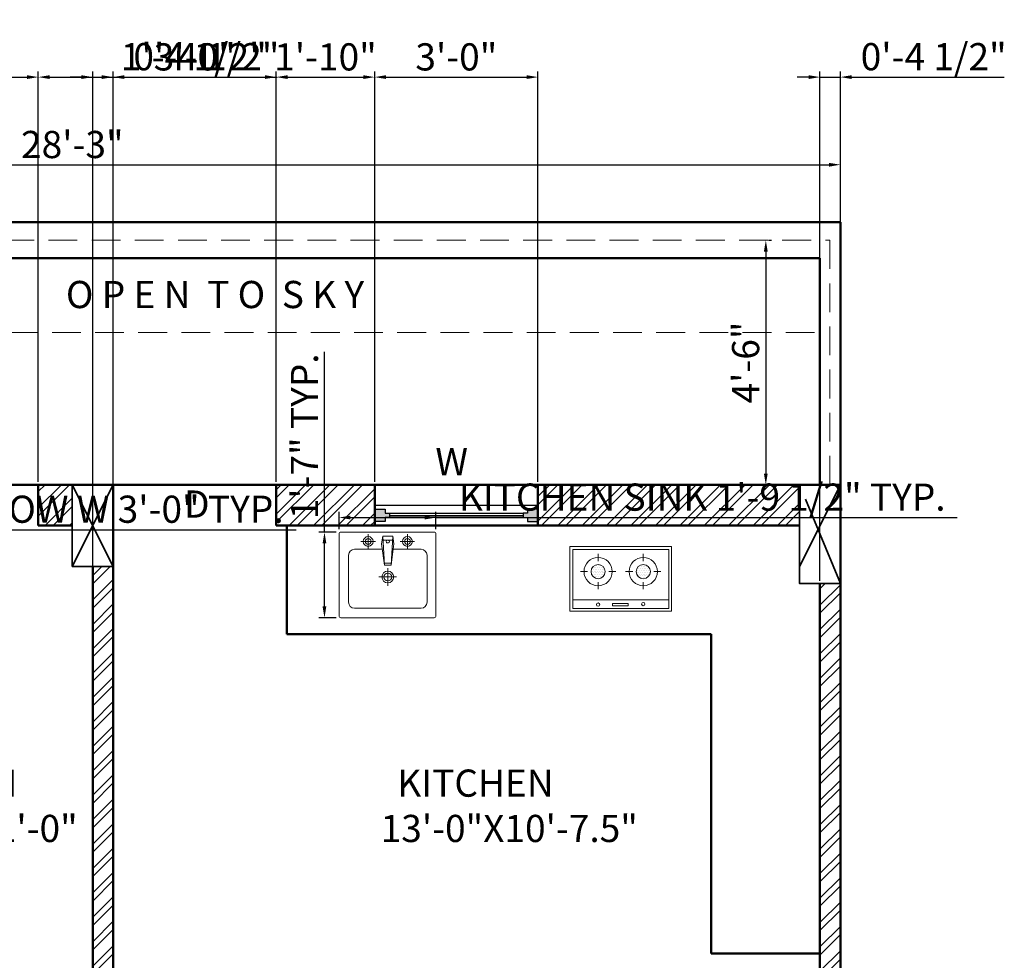
# Model space of a CAD drawing. Units: millimetres. Extents: x 67033 to 68301, y 155969 to 157209.
# Tile 6 of 17: x 67226 to 67444, y 156978 to 157186. Entities that reach past the tile are written whole.
import ezdxf

# ---------------------------------------------------------------- set-up
doc = ezdxf.new("R2010")
doc.units = ezdxf.units.MM
doc.linetypes.add('HIDDEN', pattern=[9.525, 6.35, -3.175])
for name, color, linetype, lineweight in [('A-ANNO-DIMS', 2, 'Continuous', 18), ('A-ANNO-TEXT', 7, 'Continuous', 18), ('A-AREA-IDEN', 3, 'Continuous', 18), ('A-COLS', 3, 'Continuous', 35), ('A-FLOR-FIXT', 9, 'Continuous', 18), ('A-FLOR-OVHD', 1, 'HIDDEN', 18), ('A-GLAZ', 4, 'Continuous', 25), ('A-WALL', 7, 'Continuous', 50), ('A-WALL-PATT', 8, 'Continuous', 13)]:
    doc.layers.add(name, color=color, linetype=linetype, lineweight=lineweight)
doc.styles.get("Standard").update_dxf_attribs({"font": 'arial.ttf'})
doc.dimstyles.new('ISO-25', dxfattribs={"dimtxt": 6, "dimasz": 2.5, "dimexe": 1.25, "dimexo": 0.625, "dimtad": 1, "dimdec": 0, "dimlunit": 3, "dimtxsty": 'Standard', "dimcen": 2.5, "dimadec": 0, "dimazin": 0, "dimtfac": 1, "dimtdec": 0, "dimtmove": 0, "dimatfit": 3, "dimfxl": 1, "dimarcsym": 0})

# ---------------------------------------------------------------- blocks, each defined once
blk = doc.blocks.new('A$C635F4E63')
for p, q in [((0, 10), (0, 426.6)), ((10, 436.6), (483.9, 436.6)), ((148.5, 425.2), (148.5, 352.2)), ((223.5, 415), (217, 376.2)), ((223.5, 415), (248.5, 415)), ((223.5, 415), (231.8, 268.5)), ((273.5, 415), (248.5, 415)), ((273.5, 415), (265.2, 268.5)), ((273.5, 415), (279.9, 376.2)), ((348.5, 425.2), (348.5, 352.2)), ((493.9, 426.6), (493.9, 10)), ((111.9, 388.7), (185, 388.7)), ((217, 376.2), (231.8, 268.5)), ((224.6, 395.4), (248.5, 395.4)), ((272.3, 395.4), (248.5, 395.4)), ((279.9, 376.2), (265.2, 268.5)), ((311.9, 388.7), (385, 388.7)), ((48.5, 318.8), (48.5, 78.8)), ((220.8, 348.8), (78.5, 348.8)), ((418.5, 348.8), (276.2, 348.8)), ((448.5, 318.8), (448.5, 78.8)), ((231.3, 278.6), (248.5, 278.6)), ((231.8, 268.5), (248.5, 268.5)), ((265.6, 278.6), (248.5, 278.6)), ((265.2, 268.5), (248.5, 268.5)), ((248.5, 252.8), (248.5, 162.6)), ((203.4, 207.7), (293.5, 207.7)), ((418.5, 48.8), (78.5, 48.8)), ((483.9, 0), (10, 0))]:
    blk.add_line(p, q)
for centre, radius in [((148.5, 388.7), 25), ((148.5, 388.7), 15), ((348.5, 388.7), 25), ((348.5, 388.7), 15), ((248.5, 207.7), 30), ((248.5, 207.7), 20)]:
    blk.add_circle(centre, radius)
for centre, radius, start, end in [((10, 426.6), 10, 90, 180), ((483.9, 426.6), 10, 0, 90), ((247.3, 388), 7.19, 80.5252, 279.4748), ((249.6, 388), 7.19, 260.5252, 99.4748), ((78.5, 318.8), 30, 90, 180), ((418.5, 318.8), 30, 0, 90), ((78.5, 78.8), 30, 180, 270), ((418.5, 78.8), 30, 270, 0), ((10, 10), 10, 180, 270), ((483.9, 10), 10, 270, 0)]:
    blk.add_arc(centre, radius, start, end)
blk = doc.blocks.new('A$C475E21CF')
for p, q in [((0, 444.5), (0, 0)), ((0, 444.5), (699.9, 444.5)), ((19.4, 425), (19.4, 19.4)), ((19.4, 425), (680.5, 425)), ((680.5, 425), (680.5, 19.4)), ((699.9, 444.5), (699.9, 0)), ((194.5, 393.9), (194.5, 345.2)), ((505.4, 393.9), (505.4, 345.2)), ((72.9, 272.3), (121.6, 272.3)), ((154.8, 276.2), (154.8, 276.2)), ((160.9, 288.4), (160.9, 288.4)), ((166.9, 300.5), (166.9, 300.5)), ((166.9, 276.2), (166.9, 276.2)), ((173, 288.4), (173, 288.4)), ((179.1, 300.5), (179.1, 300.5)), ((179.1, 276.2), (179.1, 276.2)), ((185.2, 312.7), (185.2, 312.7)), ((185.2, 288.4), (185.2, 288.4)), ((191.2, 300.5), (191.2, 300.5)), ((191.2, 276.2), (191.2, 276.2)), ((197.3, 312.7), (197.3, 312.7)), ((197.3, 288.4), (197.3, 288.4)), ((203.4, 300.5), (203.4, 300.5)), ((203.4, 276.2), (203.4, 276.2)), ((209.5, 312.7), (209.5, 312.7)), ((209.5, 288.4), (209.5, 288.4)), ((215.6, 300.5), (215.6, 300.5)), ((215.6, 276.2), (215.6, 276.2)), ((221.6, 288.4), (221.6, 288.4)), ((227.7, 300.5), (227.7, 300.5)), ((227.7, 276.2), (227.7, 276.2)), ((233.8, 288.4), (233.8, 288.4)), ((239.9, 276.2), (239.9, 276.2)), ((267.4, 272.3), (316, 272.3)), ((383.9, 272.3), (432.5, 272.3)), ((468, 280.2), (468, 280.2)), ((474.1, 292.3), (474.1, 292.3)), ((480.2, 304.5), (480.2, 304.5)), ((480.2, 280.2), (480.2, 280.2)), ((486.3, 292.3), (486.3, 292.3)), ((492.3, 304.5), (492.3, 304.5)), ((492.3, 280.2), (492.3, 280.2)), ((498.4, 316.6), (498.4, 316.6)), ((498.4, 292.3), (498.4, 292.3)), ((504.5, 304.5), (504.5, 304.5)), ((504.5, 280.2), (504.5, 280.2)), ((510.6, 316.6), (510.6, 316.6)), ((510.6, 292.3), (510.6, 292.3)), ((516.7, 304.5), (516.7, 304.5)), ((516.7, 280.2), (516.7, 280.2)), ((522.7, 316.6), (522.7, 316.6)), ((522.7, 292.3), (522.7, 292.3)), ((528.8, 304.5), (528.8, 304.5)), ((528.8, 280.2), (528.8, 280.2)), ((534.9, 292.3), (534.9, 292.3)), ((541, 304.5), (541, 304.5)), ((541, 280.2), (541, 280.2)), ((547, 292.3), (547, 292.3)), ((553.1, 280.2), (553.1, 280.2)), ((578.4, 272.3), (627, 272.3)), ((148.7, 264.1), (148.7, 264.1)), ((154.8, 251.9), (154.8, 251.9)), ((160.9, 264.1), (160.9, 264.1)), ((160.9, 239.8), (160.9, 239.8)), ((166.9, 251.9), (166.9, 251.9)), ((173, 264.1), (173, 264.1)), ((173, 239.8), (173, 239.8)), ((179.1, 251.9), (179.1, 251.9)), ((179.1, 227.6), (179.1, 227.6)), ((185.2, 264.1), (185.2, 264.1)), ((185.2, 239.8), (185.2, 239.8)), ((191.2, 251.9), (191.2, 251.9)), ((191.2, 227.6), (191.2, 227.6)), ((197.3, 264.1), (197.3, 264.1)), ((197.3, 239.8), (197.3, 239.8)), ((203.4, 251.9), (203.4, 251.9)), ((203.4, 227.6), (203.4, 227.6)), ((209.5, 264.1), (209.5, 264.1)), ((209.5, 239.8), (209.5, 239.8)), ((215.6, 251.9), (215.6, 251.9)), ((215.6, 227.6), (215.6, 227.6)), ((221.6, 264.1), (221.6, 264.1)), ((221.6, 239.8), (221.6, 239.8)), ((227.7, 251.9), (227.7, 251.9)), ((233.8, 264.1), (233.8, 264.1)), ((233.8, 239.8), (233.8, 239.8)), ((239.9, 251.9), (239.9, 251.9)), ((462, 268), (462, 268)), ((468, 255.9), (468, 255.9)), ((474.1, 268), (474.1, 268)), ((474.1, 243.7), (474.1, 243.7)), ((480.2, 255.9), (480.2, 255.9)), ((486.3, 268), (486.3, 268)), ((486.3, 243.7), (486.3, 243.7)), ((492.3, 255.9), (492.3, 255.9)), ((492.3, 231.5), (492.3, 231.5)), ((498.4, 268), (498.4, 268)), ((498.4, 243.7), (498.4, 243.7)), ((504.5, 255.9), (504.5, 255.9)), ((504.5, 231.5), (504.5, 231.5)), ((510.6, 268), (510.6, 268)), ((510.6, 243.7), (510.6, 243.7)), ((516.7, 255.9), (516.7, 255.9)), ((516.7, 231.5), (516.7, 231.5)), ((522.7, 268), (522.7, 268)), ((522.7, 243.7), (522.7, 243.7)), ((528.8, 255.9), (528.8, 255.9)), ((528.8, 231.5), (528.8, 231.5)), ((534.9, 268), (534.9, 268)), ((534.9, 243.7), (534.9, 243.7)), ((541, 255.9), (541, 255.9)), ((547, 268), (547, 268)), ((547, 243.7), (547, 243.7)), ((553.1, 255.9), (553.1, 255.9)), ((194.5, 199.4), (194.5, 150.8)), ((505.4, 199.4), (505.4, 150.8)), ((19.4, 77.8), (680.5, 77.8)), ((0, 0), (699.9, 0)), ((19.4, 19.4), (680.5, 19.4)), ((293.4, 51.9), (400.6, 51.9)), ((293.4, 36.5), (293.4, 51.9)), ((400.6, 36.5), (293.4, 36.5)), ((400.6, 51.9), (400.6, 36.5))]:
    blk.add_line(p, q)
for centre, radius in [((194.5, 272.3), 97.2), ((505.4, 272.3), 97.2), ((194.5, 272.3), 48.6), ((505.4, 272.3), 48.6), ((193.9, 45.1), 11.7), ((505.2, 48.5), 11.7)]:
    blk.add_circle(centre, radius)
blk = doc.blocks.new('*D29')
at = {"layer": 'A-ANNO-DIMS', "color": 0, "lineweight": -2, "transparency": 16777216}
for p, q in [((67391.61, 157136.99), (67392.24, 157136.99)), ((67390.99, 157134.49), (67390.99, 157085.49)), ((67391.61, 157082.99), (67392.24, 157082.99))]:
    blk.add_line(p, q, dxfattribs=at)
at = {"layer": 'A-ANNO-DIMS', "color": 0, "transparency": 16777216}
for points in [[(67390.57, 157134.49), (67391.4, 157134.49), (67390.99, 157136.99)], [(67390.57, 157085.49), (67391.4, 157085.49), (67390.99, 157082.99)]]:
    blk.add_solid(points, dxfattribs=at)
at = {"layer": 'Defpoints', "color": 0, "transparency": 16777216}
for p in [(67390.99, 157136.99), (67390.99, 157082.99), (67390.99, 157082.99)]:
    blk.add_point(p, dxfattribs=at)
at = {"layer": 'A-ANNO-DIMS', "color": 0, "transparency": 16777216, "insert": (67387.3, 157109.99), "char_height": 6, "attachment_point": 5, "rotation": 90}
blk.add_mtext('4\'-6"', dxfattribs=at)
blk = doc.blocks.new('*D30')
at = {"layer": 'A-ANNO-DIMS', "color": 0, "lineweight": -2, "transparency": 16777216}
for p, q in [((67068.44, 157137.62), (67068.44, 157154.9)), ((67407.44, 157137.82), (67407.44, 157154.9)), ((67070.94, 157153.65), (67404.94, 157153.65))]:
    blk.add_line(p, q, dxfattribs=at)
at = {"layer": 'A-ANNO-DIMS', "color": 0, "transparency": 16777216}
for points in [[(67070.94, 157154.06), (67070.94, 157153.23), (67068.44, 157153.65)], [(67404.94, 157154.06), (67404.94, 157153.23), (67407.44, 157153.65)]]:
    blk.add_solid(points, dxfattribs=at)
at = {"layer": 'Defpoints', "color": 0, "transparency": 16777216}
for p in [(67407.44, 157153.65), (67068.44, 157136.99), (67407.44, 157137.19)]:
    blk.add_point(p, dxfattribs=at)
at = {"layer": 'A-ANNO-DIMS', "color": 0, "transparency": 16777216, "insert": (67237.94, 157157.34), "char_height": 6, "attachment_point": 5}
blk.add_mtext('28\'-3"', dxfattribs=at)
blk = doc.blocks.new('WIN-900')
for p, q in [((3.67, 3.22), (33.2, 3.22)), ((3.67, 2.74), (33.2, 2.74)), ((33.2, 2.27), (3.67, 2.27))]:
    blk.add_line(p, q)
blk.add_lwpolyline([(0.44, 4.99), (36.44, 4.99), (36.44, 0.49), (0.44, 0.49)], close=True)
for points in [[(0.44, 4.09), (2.73, 4.09), (2.73, 3.22), (3.67, 3.22), (3.67, 2.27), (2.73, 2.27), (2.73, 1.4), (0.44, 1.4)], [(36.44, 4.09), (34.14, 4.09), (34.14, 3.22), (33.2, 3.22), (33.2, 2.27), (34.14, 2.27), (34.14, 1.4), (36.44, 1.4)]]:
    blk.add_lwpolyline(points)
blk = doc.blocks.new('COLUMN-230x460')
for p, q in [((0.44, 17.99), (9.44, -0.01)), ((9.44, 17.99), (0.44, -0.01))]:
    blk.add_line(p, q)
blk.add_lwpolyline([(0.44, 17.99), (9.44, 17.99), (9.44, -0.01), (0.44, -0.01)], close=True)
blk = doc.blocks.new('*D51')
at = {"layer": 'A-ANNO-DIMS', "color": 0, "lineweight": -2, "transparency": 16777216}
for p, q in [((67161.44, 157077.87), (67161.44, 157071.84)), ((67197.44, 157077.87), (67197.44, 157071.84)), ((67163.94, 157073.09), (67194.94, 157073.09)), ((67197.44, 157073.09), (67287.35, 157073.09))]:
    blk.add_line(p, q, dxfattribs=at)
at = {"layer": 'A-ANNO-DIMS', "color": 0, "transparency": 16777216}
for points in [[(67163.94, 157073.51), (67163.94, 157072.68), (67161.44, 157073.09)], [(67194.94, 157073.51), (67194.94, 157072.68), (67197.44, 157073.09)]]:
    blk.add_solid(points, dxfattribs=at)
at = {"layer": 'Defpoints', "color": 0, "transparency": 16777216}
for p in [(67161.44, 157078.49), (67197.44, 157078.49), (67197.44, 157073.09)]:
    blk.add_point(p, dxfattribs=at)
at = {"layer": 'A-ANNO-DIMS', "color": 0, "transparency": 16777216, "insert": (67243.64, 157076.83), "char_height": 6, "attachment_point": 5}
blk.add_mtext('WINDOW W 3\'-0" TYP.', dxfattribs=at)
blk = doc.blocks.new('*D61')
at = {"layer": 'A-ANNO-DIMS', "color": 0, "lineweight": -2, "transparency": 16777216}
for p, q in [((67296.8, 157073.18), (67296.8, 157077.02)), ((67299.3, 157075.77), (67315.69, 157075.77)), ((67318.19, 157073.18), (67318.19, 157077.02)), ((67318.19, 157075.77), (67433.24, 157075.77))]:
    blk.add_line(p, q, dxfattribs=at)
at = {"layer": 'A-ANNO-DIMS', "color": 0, "transparency": 16777216}
for points in [[(67299.3, 157076.18), (67299.3, 157075.35), (67296.8, 157075.77)], [(67315.69, 157076.18), (67315.69, 157075.35), (67318.19, 157075.77)]]:
    blk.add_solid(points, dxfattribs=at)
at = {"layer": 'Defpoints', "color": 0, "transparency": 16777216}
for p in [(67318.19, 157075.77), (67296.8, 157072.56), (67318.19, 157072.56)]:
    blk.add_point(p, dxfattribs=at)
at = {"layer": 'A-ANNO-DIMS', "color": 0, "transparency": 16777216, "insert": (67376.96, 157079.5), "char_height": 6, "attachment_point": 5}
blk.add_mtext('KITCHEN SINK 1\'-9 1/2" TYP.', dxfattribs=at)
blk = doc.blocks.new('*D62')
at = {"layer": 'A-ANNO-DIMS', "color": 0, "lineweight": -2, "transparency": 16777216}
for p, q in [((67293.59, 157072.56), (67293.59, 157112.32)), ((67296.17, 157072.56), (67292.34, 157072.56)), ((67293.59, 157056.15), (67293.59, 157070.06)), ((67296.17, 157053.65), (67292.34, 157053.65))]:
    blk.add_line(p, q, dxfattribs=at)
at = {"layer": 'A-ANNO-DIMS', "color": 0, "transparency": 16777216}
for points in [[(67293.17, 157070.06), (67294, 157070.06), (67293.59, 157072.56)], [(67293.17, 157056.15), (67294, 157056.15), (67293.59, 157053.65)]]:
    blk.add_solid(points, dxfattribs=at)
at = {"layer": 'Defpoints', "color": 0, "transparency": 16777216}
for p in [(67293.59, 157072.56), (67296.8, 157072.56), (67296.8, 157053.65)]:
    blk.add_point(p, dxfattribs=at)
at = {"layer": 'A-ANNO-DIMS', "color": 0, "transparency": 16777216, "insert": (67289.95, 157093.69), "char_height": 6, "attachment_point": 5, "rotation": 90}
blk.add_mtext('1\'-7" TYP.', dxfattribs=at)
blk = doc.blocks.new('*D81')
at = {"layer": 'A-ANNO-DIMS', "color": 0, "lineweight": -2, "transparency": 16777216}
for p, q in [((67197.44, 157083.62), (67197.44, 157174.24)), ((67230.44, 157083.62), (67230.44, 157174.24)), ((67199.94, 157172.99), (67227.94, 157172.99))]:
    blk.add_line(p, q, dxfattribs=at)
at = {"layer": 'A-ANNO-DIMS', "color": 0, "transparency": 16777216}
for points in [[(67199.94, 157173.41), (67199.94, 157172.58), (67197.44, 157172.99)], [(67227.94, 157173.41), (67227.94, 157172.58), (67230.44, 157172.99)]]:
    blk.add_solid(points, dxfattribs=at)
at = {"layer": 'Defpoints', "color": 0, "transparency": 16777216}
for p in [(67230.44, 157172.99), (67197.44, 157082.99), (67230.44, 157082.99)]:
    blk.add_point(p, dxfattribs=at)
at = {"layer": 'A-ANNO-DIMS', "color": 0, "transparency": 16777216, "insert": (67213.94, 157176.68), "char_height": 6, "attachment_point": 5}
blk.add_mtext('2\'-9"', dxfattribs=at)
blk = doc.blocks.new('*D82')
at = {"layer": 'A-ANNO-DIMS', "color": 0, "lineweight": -2, "transparency": 16777216}
for p, q in [((67230.44, 157083.62), (67230.44, 157174.24)), ((67246.94, 157083.62), (67246.94, 157174.24)), ((67232.94, 157172.99), (67244.44, 157172.99)), ((67246.94, 157172.99), (67280.05, 157172.99))]:
    blk.add_line(p, q, dxfattribs=at)
at = {"layer": 'A-ANNO-DIMS', "color": 0, "transparency": 16777216}
for points in [[(67232.94, 157173.41), (67232.94, 157172.58), (67230.44, 157172.99)], [(67244.44, 157173.41), (67244.44, 157172.58), (67246.94, 157172.99)]]:
    blk.add_solid(points, dxfattribs=at)
at = {"layer": 'Defpoints', "color": 0, "transparency": 16777216}
for p in [(67246.94, 157172.99), (67230.44, 157082.99), (67246.94, 157082.99)]:
    blk.add_point(p, dxfattribs=at)
at = {"layer": 'A-ANNO-DIMS', "color": 0, "transparency": 16777216, "insert": (67264.74, 157176.72), "char_height": 6, "attachment_point": 5}
blk.add_mtext('1\'-4 1/2"', dxfattribs=at)
blk = doc.blocks.new('*D83')
at = {"layer": 'A-ANNO-DIMS', "color": 0, "lineweight": -2, "transparency": 16777216}
for p, q in [((67246.94, 157083.62), (67246.94, 157174.24)), ((67282.94, 157083.62), (67282.94, 157174.24)), ((67249.44, 157172.99), (67280.44, 157172.99))]:
    blk.add_line(p, q, dxfattribs=at)
at = {"layer": 'A-ANNO-DIMS', "color": 0, "transparency": 16777216}
for points in [[(67249.44, 157173.41), (67249.44, 157172.58), (67246.94, 157172.99)], [(67280.44, 157173.41), (67280.44, 157172.58), (67282.94, 157172.99)]]:
    blk.add_solid(points, dxfattribs=at)
at = {"layer": 'Defpoints', "color": 0, "transparency": 16777216}
for p in [(67282.94, 157172.99), (67246.94, 157082.99), (67282.94, 157082.99)]:
    blk.add_point(p, dxfattribs=at)
at = {"layer": 'A-ANNO-DIMS', "color": 0, "transparency": 16777216, "insert": (67264.94, 157176.68), "char_height": 6, "attachment_point": 5}
blk.add_mtext('3\'-0"', dxfattribs=at)
blk = doc.blocks.new('*D84')
at = {"layer": 'A-ANNO-DIMS', "color": 0, "lineweight": -2, "transparency": 16777216}
for p, q in [((67282.94, 157083.62), (67282.94, 157174.24)), ((67304.69, 157083.62), (67304.69, 157174.24)), ((67285.44, 157172.99), (67302.19, 157172.99))]:
    blk.add_line(p, q, dxfattribs=at)
at = {"layer": 'A-ANNO-DIMS', "color": 0, "transparency": 16777216}
for points in [[(67285.44, 157173.41), (67285.44, 157172.58), (67282.94, 157172.99)], [(67302.19, 157173.41), (67302.19, 157172.58), (67304.69, 157172.99)]]:
    blk.add_solid(points, dxfattribs=at)
at = {"layer": 'Defpoints', "color": 0, "transparency": 16777216}
for p in [(67304.69, 157172.99), (67282.94, 157082.99), (67304.69, 157082.99)]:
    blk.add_point(p, dxfattribs=at)
at = {"layer": 'A-ANNO-DIMS', "color": 0, "transparency": 16777216, "insert": (67293.81, 157176.68), "char_height": 6, "attachment_point": 5}
blk.add_mtext('1\'-10"', dxfattribs=at)
blk = doc.blocks.new('*D85')
at = {"layer": 'A-ANNO-DIMS', "color": 0, "lineweight": -2, "transparency": 16777216}
for p, q in [((67304.69, 157083.62), (67304.69, 157174.24)), ((67340.69, 157083.62), (67340.69, 157174.24)), ((67307.19, 157172.99), (67338.19, 157172.99))]:
    blk.add_line(p, q, dxfattribs=at)
at = {"layer": 'A-ANNO-DIMS', "color": 0, "transparency": 16777216}
for points in [[(67307.19, 157173.41), (67307.19, 157172.58), (67304.69, 157172.99)], [(67338.19, 157173.41), (67338.19, 157172.58), (67340.69, 157172.99)]]:
    blk.add_solid(points, dxfattribs=at)
at = {"layer": 'Defpoints', "color": 0, "transparency": 16777216}
for p in [(67340.69, 157172.99), (67304.69, 157082.99), (67340.69, 157082.99)]:
    blk.add_point(p, dxfattribs=at)
at = {"layer": 'A-ANNO-DIMS', "color": 0, "transparency": 16777216, "insert": (67322.69, 157176.68), "char_height": 6, "attachment_point": 5}
blk.add_mtext('3\'-0"', dxfattribs=at)
blk = doc.blocks.new('*D93')
at = {"layer": 'A-ANNO-DIMS', "color": 0, "lineweight": -2, "transparency": 16777216}
for p, q in [((67242.44, 156960.62), (67242.44, 157174.24)), ((67246.94, 156960.62), (67246.94, 157174.24)), ((67239.94, 157172.99), (67237.44, 157172.99)), ((67242.44, 157172.99), (67246.94, 157172.99)), ((67249.44, 157172.99), (67283.12, 157172.99))]:
    blk.add_line(p, q, dxfattribs=at)
at = {"layer": 'A-ANNO-DIMS', "color": 0, "transparency": 16777216}
for points in [[(67239.94, 157173.41), (67239.94, 157172.58), (67242.44, 157172.99)], [(67249.44, 157173.41), (67249.44, 157172.58), (67246.94, 157172.99)]]:
    blk.add_solid(points, dxfattribs=at)
at = {"layer": 'Defpoints', "color": 0, "transparency": 16777216}
for p in [(67246.94, 157172.99), (67242.44, 156959.99), (67246.94, 156959.99)]:
    blk.add_point(p, dxfattribs=at)
at = {"layer": 'A-ANNO-DIMS', "color": 0, "transparency": 16777216, "insert": (67267.53, 157176.72), "char_height": 6, "attachment_point": 5}
blk.add_mtext('0\'-4 1/2"', dxfattribs=at)
blk = doc.blocks.new('*D94')
at = {"layer": 'A-ANNO-DIMS', "color": 0, "lineweight": -2, "transparency": 16777216}
for p, q in [((67402.94, 157061.82), (67402.94, 157174.24)), ((67407.44, 157061.82), (67407.44, 157174.24)), ((67400.44, 157172.99), (67397.94, 157172.99)), ((67402.94, 157172.99), (67407.44, 157172.99)), ((67409.94, 157172.99), (67443.62, 157172.99))]:
    blk.add_line(p, q, dxfattribs=at)
at = {"layer": 'A-ANNO-DIMS', "color": 0, "transparency": 16777216}
for points in [[(67400.44, 157173.41), (67400.44, 157172.58), (67402.94, 157172.99)], [(67409.94, 157173.41), (67409.94, 157172.58), (67407.44, 157172.99)]]:
    blk.add_solid(points, dxfattribs=at)
at = {"layer": 'Defpoints', "color": 0, "transparency": 16777216}
for p in [(67407.44, 157172.99), (67402.94, 157061.19), (67407.44, 157061.19)]:
    blk.add_point(p, dxfattribs=at)
at = {"layer": 'A-ANNO-DIMS', "color": 0, "transparency": 16777216, "insert": (67428.03, 157176.72), "char_height": 6, "attachment_point": 5}
blk.add_mtext('0\'-4 1/2"', dxfattribs=at)

msp = doc.modelspace()

# ---------------------------------------------------------------- hatches: boundary and pattern name
at = {"layer": 'A-GLAZ'}
h = msp.add_hatch(color=256, dxfattribs=at)
h.dxf.hatch_style = 1
h.paths.add_polyline_path([(67307.92, 157076.72), (67306.98, 157076.72), (67306.98, 157077.59), (67304.69, 157077.59), (67304.69, 157074.9), (67306.98, 157074.9), (67306.98, 157075.77), (67307.92, 157075.77)])
h = msp.add_hatch(color=256, dxfattribs=at)
h.dxf.hatch_style = 1
h.paths.add_polyline_path([(67340.69, 157077.59), (67338.39, 157077.59), (67338.39, 157076.72), (67337.45, 157076.72), (67337.45, 157075.77), (67338.39, 157075.77), (67338.39, 157074.9), (67340.69, 157074.9)])
at = {"layer": 'A-WALL-PATT'}
h = msp.add_hatch(dxfattribs=at)
h.set_pattern_fill('ANSI32', color=256, scale=0.4)
h.paths.add_polyline_path([(67237.94, 157082.99), (67230.44, 157082.99), (67230.44, 157073.99), (67237.94, 157073.99)])
h = msp.add_hatch(dxfattribs=at)
h.set_pattern_fill('ANSI32', color=256, scale=0.4)
h.paths.add_polyline_path([(67304.69, 157082.99), (67282.94, 157082.99), (67282.94, 157073.99), (67304.69, 157073.99)])
h = msp.add_hatch(dxfattribs=at)
h.set_pattern_fill('ANSI32', color=256, scale=0.4)
h.paths.add_polyline_path([(67398.44, 157082.99), (67340.69, 157082.99), (67340.69, 157073.99), (67398.44, 157073.99)])
h = msp.add_hatch(dxfattribs=at)
h.set_pattern_fill('ANSI32', color=256, scale=0.4)
h.paths.add_polyline_path([(67246.94, 157064.99), (67242.44, 157064.99), (67242.44, 156959.99), (67246.94, 156959.99)])
h = msp.add_hatch(dxfattribs=at)
h.set_pattern_fill('ANSI32', color=256, scale=0.4)
h.paths.add_polyline_path([(67407.44, 157061.19), (67402.94, 157061.19), (67402.94, 156959.99), (67407.44, 156959.99)])

# ---------------------------------------------------------------- linework, layer by layer
at = {"layer": 'A-COLS'}
for p, q in [((67407.44, 157082.99), (67398.44, 157064.99)), ((67399.76, 157079.8), (67407.44, 157061.19))]:
    msp.add_line(p, q, dxfattribs=at)
msp.add_lwpolyline([(67398.44, 157082.99), (67407.44, 157082.99), (67407.44, 157061.19), (67398.44, 157061.19)], close=True, dxfattribs=at)
at = {"layer": 'A-FLOR-OVHD'}
for p, q in [((67137.44, 157136.99), (67405.1, 157136.99)), ((67405.1, 157136.99), (67405.1, 157082.99)), ((67195.36, 157116.61), (67402.94, 157116.61))]:
    msp.add_line(p, q, dxfattribs=at)
at = {"layer": 'A-WALL'}
for p, q in [((67068.44, 157140.99), (67407.44, 157140.99)), ((67407.44, 157140.99), (67407.44, 156527.99)), ((67137.44, 157132.99), (67402.94, 157132.99)), ((67402.94, 157132.99), (67402.94, 157082.99)), ((67197.44, 157082.99), (67230.44, 157082.99)), ((67230.44, 157082.99), (67230.44, 157073.99)), ((67230.44, 157082.99), (67407.44, 157082.99)), ((67246.94, 157082.99), (67246.94, 156941.99)), ((67282.94, 157082.99), (67282.94, 157073.99)), ((67304.69, 157073.99), (67304.69, 157082.99)), ((67340.69, 157073.99), (67340.69, 157082.99)), ((67304.69, 157078.49), (67304.69, 157073.99)), ((67340.69, 157078.49), (67340.69, 157073.99)), ((67230.44, 157073.99), (67237.94, 157073.99)), ((67282.94, 157073.99), (67398.44, 157073.99)), ((67285.3, 157073.99), (67285.3, 157049.99)), ((67242.44, 157064.99), (67242.44, 156959.99)), ((67402.94, 157061.19), (67402.94, 156959.99)), ((67285.3, 157049.99), (67378.94, 157049.99)), ((67378.94, 157049.99), (67378.94, 156979.55)), ((67378.94, 156979.55), (67402.94, 156979.55))]:
    msp.add_line(p, q, dxfattribs=at)

# ---------------------------------------------------------------- block references
at = {"layer": 'A-COLS'}
msp.add_blockref('COLUMN-230x460', (67237.5, 157065), dxfattribs=at)
at = {"layer": 'A-FLOR-FIXT'}
for name, p, xscale, yscale, zscale in [('A$C635F4E63', (67296.8, 157053.65), 0.0433159964901652, 0.0433159964901652, 0.0433159964901652), ('A$C475E21CF', (67347.75, 157055.1), 0.0320579729999927, 0.0320579729999927, 0.0320579729999927)]:
    msp.add_blockref(name, p, dxfattribs=dict(at, xscale=xscale, yscale=yscale, zscale=zscale))
at = {"layer": 'A-GLAZ'}
msp.add_blockref('WIN-900', (67304.25, 157073.5), dxfattribs=at)

# ---------------------------------------------------------------- texts
at = {"layer": 'A-ANNO-TEXT', "char_height": 6, "attachment_point": 1}
for s, insert in [('   W', (67312.57, 157091.11)), ('   D', (67257.1, 157081.74))]:
    msp.add_mtext_dynamic_manual_height_columns(s, width=19.5287, gutter_width=12.5, heights=[0], dxfattribs=dict(at, insert=insert))
at = {"layer": 'A-AREA-IDEN', "char_height": 6, "attachment_point": 1}
for s, width, insert in [('              O P E N  T O  S K Y', 118.0294, (67210.86, 157128)), ('  BEDROOM \\P14\'-1.5"X11\'-0"', 59.4046, (67182.37, 157020.14)), ('  KITCHEN\\P13\'-0"X10\'-7.5"', 62.0967, (67305.99, 157020.14))]:
    msp.add_mtext_dynamic_manual_height_columns(s, width=width, gutter_width=12.5, heights=[0], dxfattribs=dict(at, insert=insert))

# ---------------------------------------------------------------- dimensions: what is measured, and where the dimension line sits
at = {"layer": 'A-ANNO-DIMS'}
for base, p1, p2, override, picture, middle in [((67246.94, 157172.99), (67230.44, 157082.99), (67246.94, 157082.99), {"dimdec": 1, "dimlfac": 1, "dimrnd": 0, "dimzin": 1, "dimdsep": 46, "dimlunit": 4, "dimfrac": 2}, '*D82', (67264.74, 157176.72)), ((67246.94, 157172.99), (67242.44, 156959.99), (67246.94, 156959.99), {"dimdec": 1, "dimlfac": 1, "dimrnd": 0, "dimzin": 1, "dimdsep": 46, "dimlunit": 4, "dimfrac": 2}, '*D93', (67267.53, 157176.72)), ((67407.44, 157172.99), (67402.94, 157061.19), (67407.44, 157061.19), {"dimdec": 1, "dimlfac": 1, "dimrnd": 0, "dimzin": 1, "dimdsep": 46, "dimlunit": 4, "dimfrac": 2}, '*D94', (67428.03, 157176.72)), ((67230.44, 157172.99), (67197.44, 157082.99), (67230.44, 157082.99), {"dimdec": 1, "dimlfac": 1, "dimrnd": 0, "dimzin": 1, "dimdsep": 46, "dimlunit": 4, "dimfrac": 2}, '*D81', (67213.94, 157176.68)), ((67282.94, 157172.99), (67246.94, 157082.99), (67282.94, 157082.99), {"dimdec": 1, "dimlfac": 1, "dimrnd": 0, "dimzin": 1, "dimdsep": 46, "dimlunit": 4, "dimfrac": 2}, '*D83', (67264.94, 157176.68)), ((67304.686587, 157172.994117), (67282.936587, 157082.994117), (67304.686587, 157082.994117), {"dimdec": 1, "dimlfac": 1, "dimrnd": 0, "dimzin": 1, "dimdsep": 46, "dimlunit": 4, "dimfrac": 2}, '*D84', (67293.811587, 157176.68255493)), ((67340.69, 157172.99), (67304.69, 157082.99), (67340.69, 157082.99), {"dimdec": 1, "dimlfac": 1, "dimrnd": 0, "dimzin": 1, "dimdsep": 46, "dimlunit": 4, "dimfrac": 2}, '*D85', (67322.69, 157176.68)), ((67407.44, 157153.65), (67068.44, 157136.99), (67407.44, 157137.19), {"dimclrd": 0, "dimclre": 0, "dimclrt": 0}, '*D30', (67237.94, 157157.34))]:
    dim = msp.add_linear_dim(base=base, p1=p1, p2=p2, dimstyle='ISO-25', override=override, dxfattribs=at)
    dim.commit()
    dim.dimension.update_dxf_attribs({"geometry": picture, "text_midpoint": middle})
dim = msp.add_linear_dim(base=(67390.99, 157082.99), p1=(67390.99, 157136.99), p2=(67390.99, 157082.99), angle=90, dimstyle='ISO-25', override={"dimclrd": 0, "dimclre": 0, "dimclrt": 0}, dxfattribs=at)
dim.commit()
dim.dimension.update_dxf_attribs({"geometry": '*D29', "text_midpoint": (67387.3, 157109.99)})
dim = msp.add_linear_dim(base=(67293.59, 157072.56), p1=(67296.8, 157053.65), p2=(67296.8, 157072.56), angle=90, text='<> TYP.', dimstyle='ISO-25', override={"dimdec": 1, "dimrnd": 0, "dimzin": 1, "dimlunit": 4, "dimfrac": 2}, dxfattribs=at)
dim.commit()
dim.dimension.update_dxf_attribs({"geometry": '*D62', "text_midpoint": (67289.95, 157093.69)})
for base, p1, p2, text, picture, middle in [((67318.19, 157075.77), (67296.8, 157072.56), (67318.19, 157072.56), 'KITCHEN SINK <> TYP.', '*D61', (67376.96, 157079.5)), ((67197.44, 157073.09), (67161.44, 157078.49), (67197.44, 157078.49), 'WINDOW W <> TYP.', '*D51', (67243.64, 157076.83))]:
    dim = msp.add_linear_dim(base=base, p1=p1, p2=p2, text=text, dimstyle='ISO-25', override={"dimdec": 1, "dimrnd": 0, "dimzin": 1, "dimlunit": 4, "dimfrac": 2}, dxfattribs=at)
    dim.commit()
    dim.dimension.update_dxf_attribs({"geometry": picture, "text_midpoint": middle})

doc.saveas('drawing.dxf')
